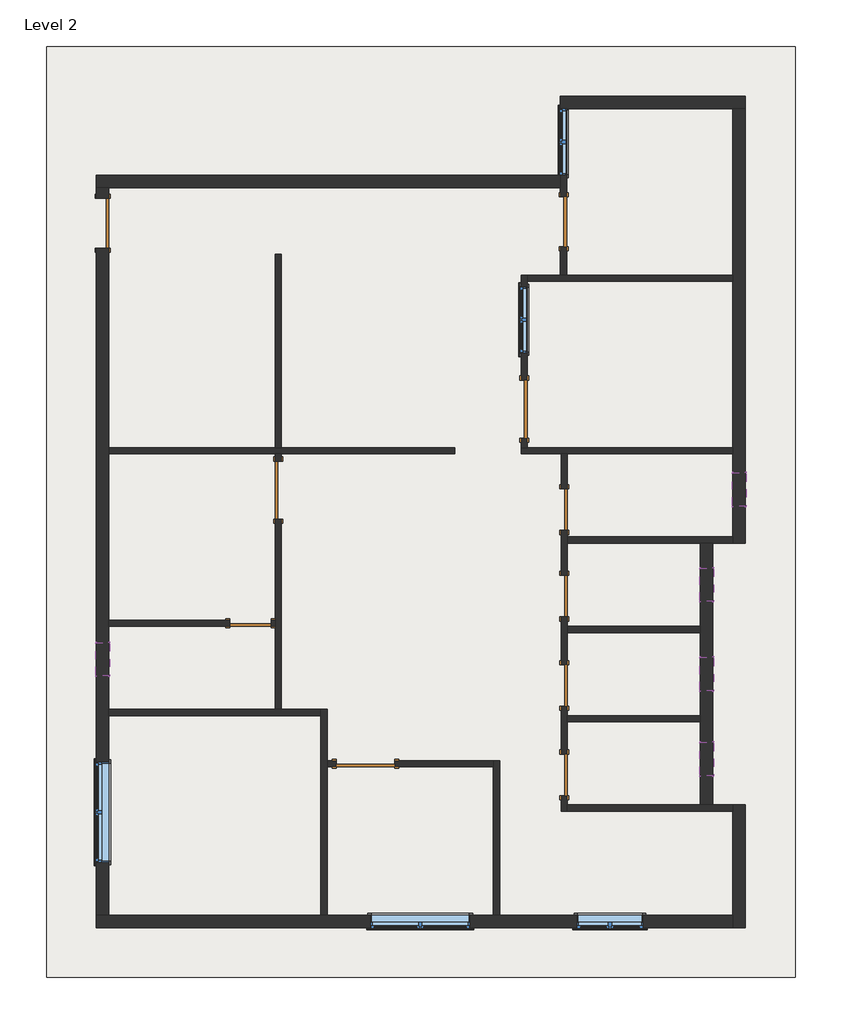
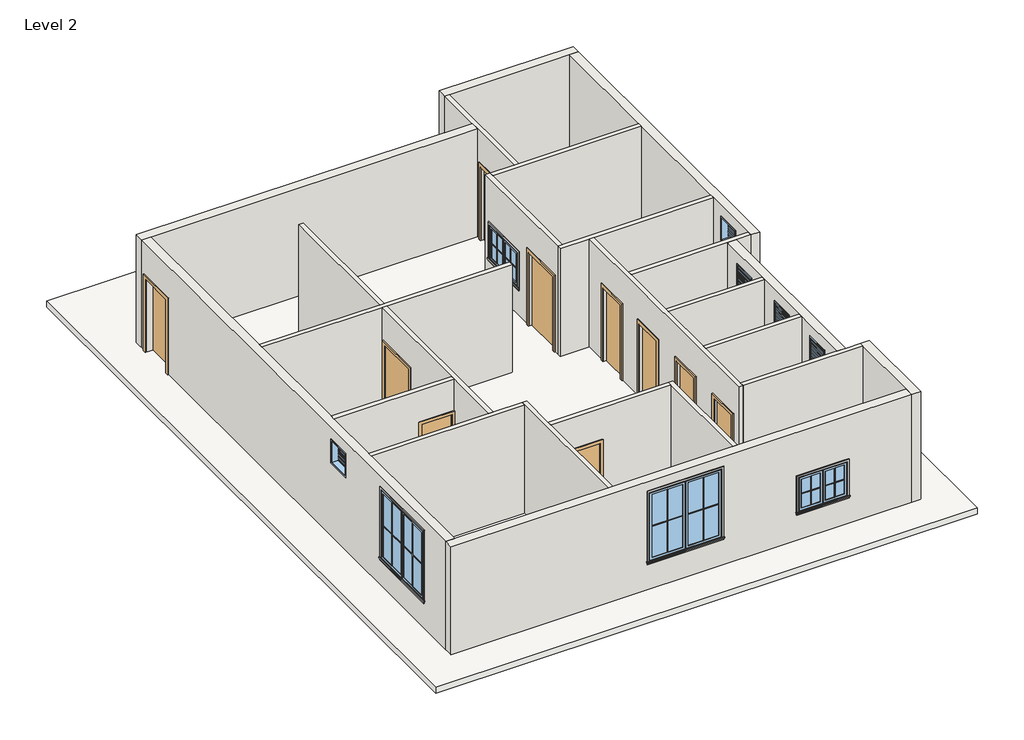
# One storey, incomplete: 23 walls, 20 proxies, 10 doors, 10 windows, 1 roof.
# Revit data of these elements (continued)
# Elements 48, 49, 50, 51, 52, 53, 54 (IfcWall, "WALL 9\"") (continued)
#   wall height = 10' - 0"
#   Phase Created = New Construction
#   Base Constraint = Level 2
#   Materials on its faces: "Default Wall", "Wood - Stained"
# Element 55 (IfcWindow, "Window-Casement-Double : WIN 4'")
#   Mark = "13"
#   Window Inset = 0' - 0"
#   Interior Wall Closure = 0' - 2 1/4"
#   Frame Extension = 0' - 0 1/4"
#   Exterior Wall Closure = 0' - 1 1/4"
#   Interior Trim Visibility = yes
#   Exterior Trim Visibility = yes
#   Phase Created = New Construction
#   Materials on its faces: "Wood - Stained", "Glass", "Clad - White"
# Element 56 (IfcWindow, "Window-Casement-Double : WIN 4'")
#   Mark = "14"
#   Window Inset = 0' - 0"
#   Interior Wall Closure = 0' - 2 1/4"
#   Frame Extension = 0' - 0 1/4"
#   Exterior Wall Closure = 0' - 1 1/4"
#   Interior Trim Visibility = yes
#   Exterior Trim Visibility = yes
#   Phase Created = New Construction
#   Materials on its faces: "Wood - Stained", "Glass", "Clad - White"
# Element 57 (IfcWindow, "Window-Casement-Double : WIN 4'")
#   Mark = "15"
#   Window Inset = 0' - 0"
#   Interior Wall Closure = 0' - 2 1/4"
#   Frame Extension = 0' - 0 1/4"
#   Exterior Wall Closure = 0' - 1 1/4"
#   Interior Trim Visibility = yes
#   Exterior Trim Visibility = yes
#   Phase Created = New Construction
#   Materials on its faces: "Wood - Stained", "Glass", "Clad - White"
# Element 58 (IfcWindow, "Window-Casement-Double : WIN 6'")
#   Mark = "11"
#   Window Inset = 0' - 0"
#   Interior Wall Closure = 0' - 2 1/4"
#   Frame Extension = 0' - 0 1/4"
#   Exterior Wall Closure = 0' - 1 1/4"
#   Interior Trim Visibility = yes
#   Exterior Trim Visibility = yes
#   Phase Created = New Construction
#   Materials on its faces: "Wood - Stained", "Glass", "Clad - White"
# Element 59 (IfcWindow, "Window-Casement-Double : WIN 6'")
#   Mark = "12"
#   Window Inset = 0' - 0"
#   Interior Wall Closure = 0' - 2 1/4"
#   Frame Extension = 0' - 0 1/4"
#   Exterior Wall Closure = 0' - 1 1/4"
#   Interior Trim Visibility = yes
#   Exterior Trim Visibility = yes
#   Phase Created = New Construction
#   Materials on its faces: "Wood - Stained", "Glass", "Clad - White"
# Element 60 (IfcWindow, "Window-Louvers : 24\" x 24\"")
#   Mark = "16"
#   Blade Width = 1' - 10 1/2"
#   Phase Created = New Construction
#   Materials on its faces: "Birch"
# Element 61 (IfcWindow, "Window-Louvers : 24\" x 24\"")
#   Mark = "17"
#   Blade Width = 1' - 10 1/2"
#   Phase Created = New Construction
#   Materials on its faces: "Birch"
# Element 62 (IfcWindow, "Window-Louvers : 24\" x 24\"")
#   Mark = "18"
#   Blade Width = 1' - 10 1/2"
#   Phase Created = New Construction
#   Materials on its faces: "Birch"
# Element 63 (IfcWindow, "Window-Louvers : 24\" x 24\"")
#   Mark = "19"
#   Blade Width = 1' - 10 1/2"
#   Phase Created = New Construction
#   Materials on its faces: "Birch"
# Element 64 (IfcWindow, "Window-Louvers : 24\" x 24\"")
#   Mark = "20"
#   Blade Width = 1' - 10 1/2"
#   Phase Created = New Construction
#   Materials on its faces: "Birch"
# Materials
#   "Door - Panel": class "Wood", colour RGB 210 159 95, transparency 0, Cost = 0
#   "Door - Frame": colour RGB 118 70 51, transparency 0, Cost = 0
#   "Wood - Stained": class "Wood", colour RGB 224 178 126, transparency 0, Cost = 0
#   "Glass": class "Glass", colour RGB 0 128 192, transparency 0.75, Description = "Soda Lime Glass", Cost = 0
#   "Clad - White": class "Wood", colour RGB 242 242 238, transparency 0, Cost = 0
#   "Birch": class "Wood", colour RGB 224 178 126, transparency 0, Description = "Betula Alleghaniensis", Cost = 0
#   "Cherry": class "Wood", colour RGB 226 177 128, transparency 0, Description = "Prunus Serotina", Cost = 0
#   "Default Roof": colour RGB 88 101 114, transparency 0, Cost = 0
#   "Wood Planks": class "Wood", colour RGB 193 160 115, transparency 0, Description = "Physical material.", Cost = 0
#   "Default Wall": colour RGB 128 128 128, transparency 0, Cost = 0
